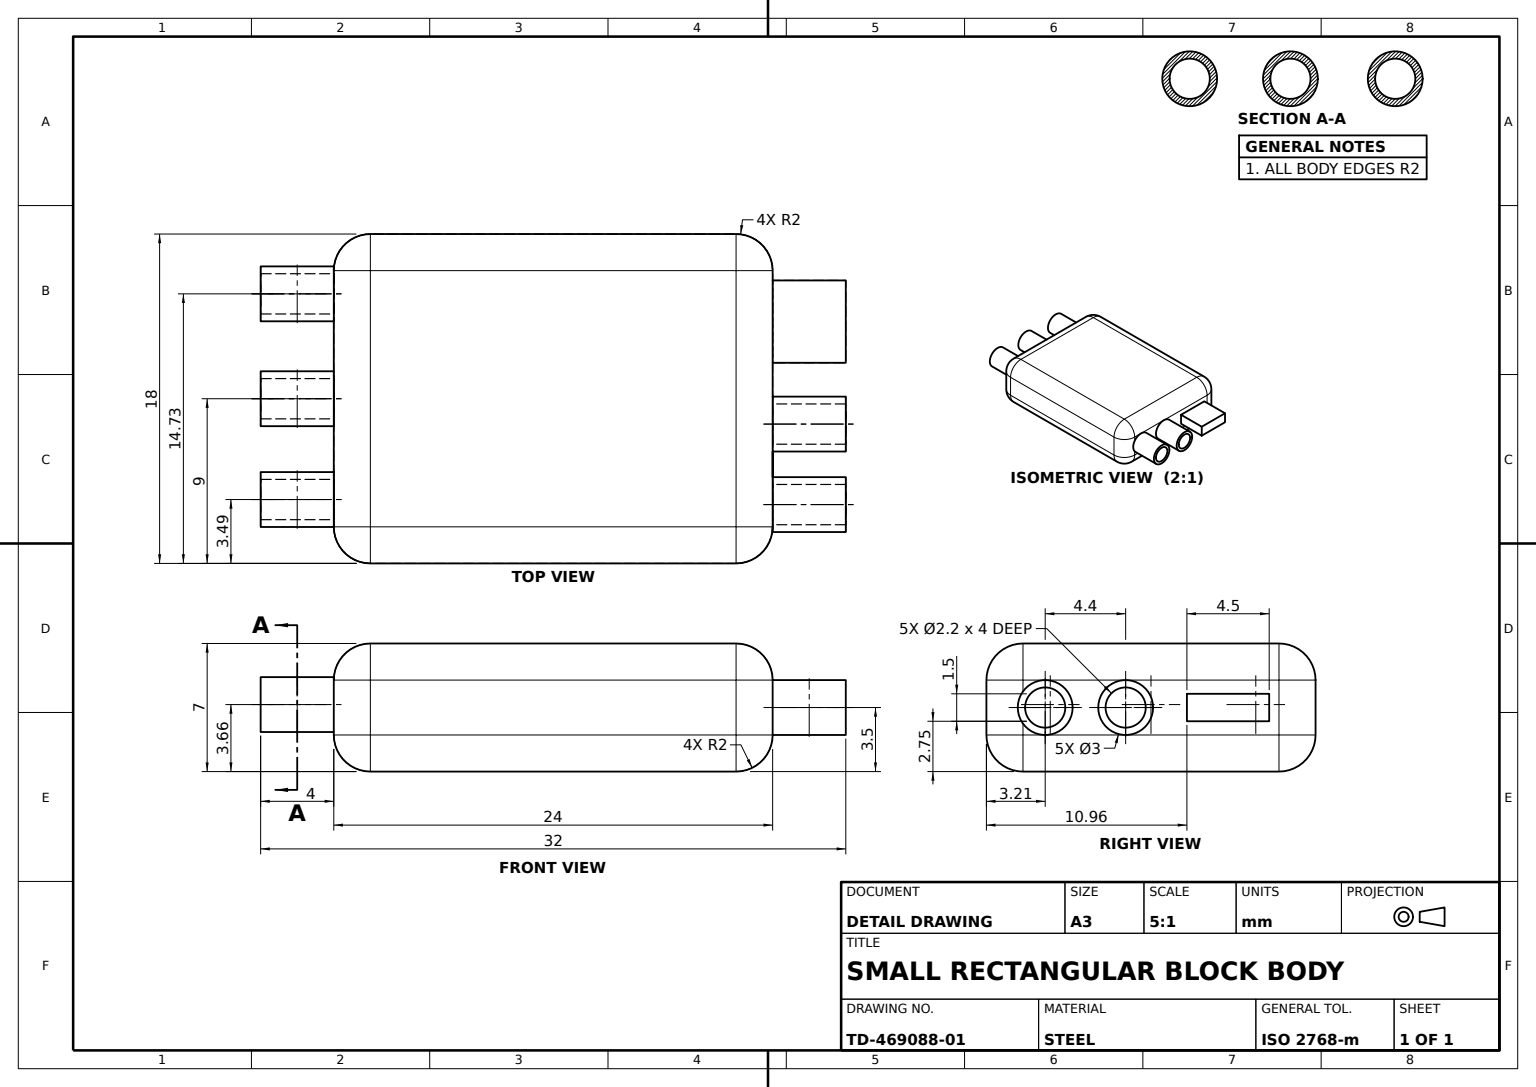
from build123d import *

# Parameters (mm, degrees)
HOUSING_BODY_DEPTH               = 7
HOUSING_EDGE_FILLET_R2_R         = 2
PIN_SET_A_SKETCH_R               = 1.5
PIN_SET_A_SKETCH_R_2             = 1.1
TUBULAR_PINS_SET_A_3_DEPTH       = 4
PIN_SET_B_AND_TAB_SKETCH_R       = 1.5
PIN_SET_B_AND_TAB_SKETCH_R_2     = 1.1
PIN_SET_B_AND_TAB_SKETCH_W       = 4.5
PIN_SET_B_AND_TAB_SKETCH_H       = 1.5
TUBULAR_PINS_SET_B_AND_TAB_DEPTH = 4


with BuildPart() as part:
    # Housing Profile Sketch → Housing Body (new body)
    with BuildSketch(Plane(origin=(0, 0, 0), x_dir=(1, 0, 0), z_dir=(0, 1, 0))):
        with BuildLine():
            Line((-10, 9), (10, 9))
            ThreePointArc((10, 9), (11.414213562, 8.414213562), (12, 7))
            Line((12, 7), (12, -7))
            ThreePointArc((12, -7), (11.414213562, -8.414213562), (10, -9))
            Line((10, -9), (-10, -9))
            ThreePointArc((-10, -9), (-11.414213562, -8.414213562), (-12, -7))
            Line((-12, -7), (-12, 7))
            ThreePointArc((-12, 7), (-11.414213562, 8.414213562), (-10, 9))
        make_face()
    extrude(amount=HOUSING_BODY_DEPTH)

    # Housing Edge Fillet R2
    housing_edge_fillet_r2_edges = [part.edges().sort_by_distance(p)[0] for p in [
        (-12, 0, 0),
        (-11.414213562, 0, -8.414213562),
        (0, 0, -9),
        (11.414213562, 0, -8.414213562),
        (-11.414213562, 7, -8.414213562),
        (-12, 7, 0),
        (-11.414213562, 7, 8.414213562),
        (0, 7, 9),
        (11.414213562, 7, 8.414213562),
        (12, 7, 0),
        (11.414213562, 7, -8.414213562),
        (12, 0, 0),
        (0, 7, -9),
        (11.414213562, 0, 8.414213562),
        (0, 0, 9),
        (-11.414213562, 0, 8.414213562),
    ]]
    fillet(housing_edge_fillet_r2_edges, radius=HOUSING_EDGE_FILLET_R2_R)

    # Pin Set A Sketch → Tubular Pins Set A Ø3 (add)
    # profile 1 of 3: a face of its own
    with BuildSketch(Plane.ZY.offset(12)):
        with Locations(Location((0, 3.661725767, 0), (0, 0, 116.851166023))):
            Circle(PIN_SET_A_SKETCH_R)
        with Locations((0, 3.661725767)):
            Circle(PIN_SET_A_SKETCH_R_2, mode=Mode.SUBTRACT)
    # profile 2 of 3: a face of its own
    with BuildSketch(Plane.ZY.offset(12)):
        with Locations(Location((-5.731156871, 3.661725767, 0), (0, 0, 212.232000091))):
            Circle(PIN_SET_A_SKETCH_R)
        with Locations((-5.731156871, 3.661725767)):
            Circle(PIN_SET_A_SKETCH_R_2, mode=Mode.SUBTRACT)
    # profile 3 of 3: a face of its own
    with BuildSketch(Plane.ZY.offset(12)):
        with Locations(Location((5.508783942, 3.661725767, 0), (0, 0, 116.851166023))):
            Circle(PIN_SET_A_SKETCH_R)
        with Locations((5.508783942, 3.661725767)):
            Circle(PIN_SET_A_SKETCH_R_2, mode=Mode.SUBTRACT)
    extrude(amount=TUBULAR_PINS_SET_A_3_DEPTH)

    # Pin Set B and Tab Sketch → Tubular Pins Set B and Tab (add)
    # profile 1 of 3: a face of its own
    with BuildSketch(Plane(origin=(12, 0, 0), x_dir=(0, 0, -1), z_dir=(1, 0, 0))):
        with Locations(Location((-5.785268851, 3.5, 0), (0, 0, 215.921576532))):
            Circle(PIN_SET_B_AND_TAB_SKETCH_R)
        with Locations((-5.785268851, 3.5)):
            Circle(PIN_SET_B_AND_TAB_SKETCH_R_2, mode=Mode.SUBTRACT)
    # profile 2 of 3: a face of its own
    with BuildSketch(Plane(origin=(12, 0, 0), x_dir=(0, 0, -1), z_dir=(1, 0, 0))):
        with Locations(Location((-1.385268851, 3.5, 0), (0, 0, 270))):
            Circle(PIN_SET_B_AND_TAB_SKETCH_R)
        with Locations((-1.385268851, 3.5)):
            Circle(PIN_SET_B_AND_TAB_SKETCH_R_2, mode=Mode.SUBTRACT)
    # profile 3 of 3: a face of its own
    with BuildSketch(Plane(origin=(12, 0, 0), x_dir=(0, 0, -1), z_dir=(1, 0, 0))):
        with Locations((4.21427792, 3.5)):
            Rectangle(PIN_SET_B_AND_TAB_SKETCH_W, PIN_SET_B_AND_TAB_SKETCH_H)
    extrude(amount=TUBULAR_PINS_SET_B_AND_TAB_DEPTH)


solid = part.part
